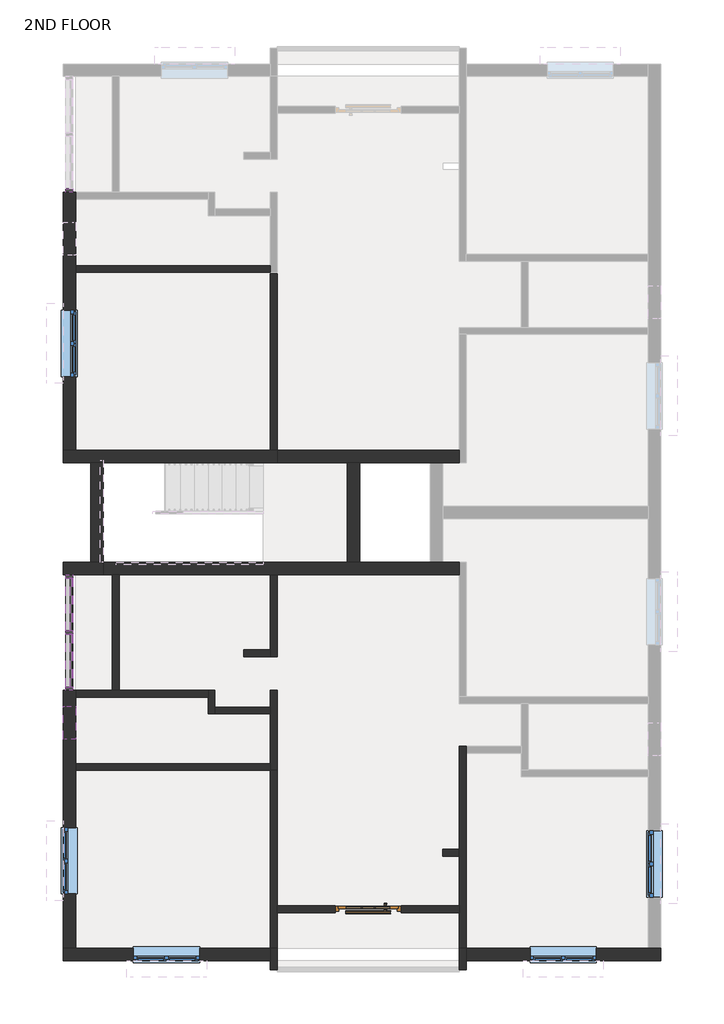
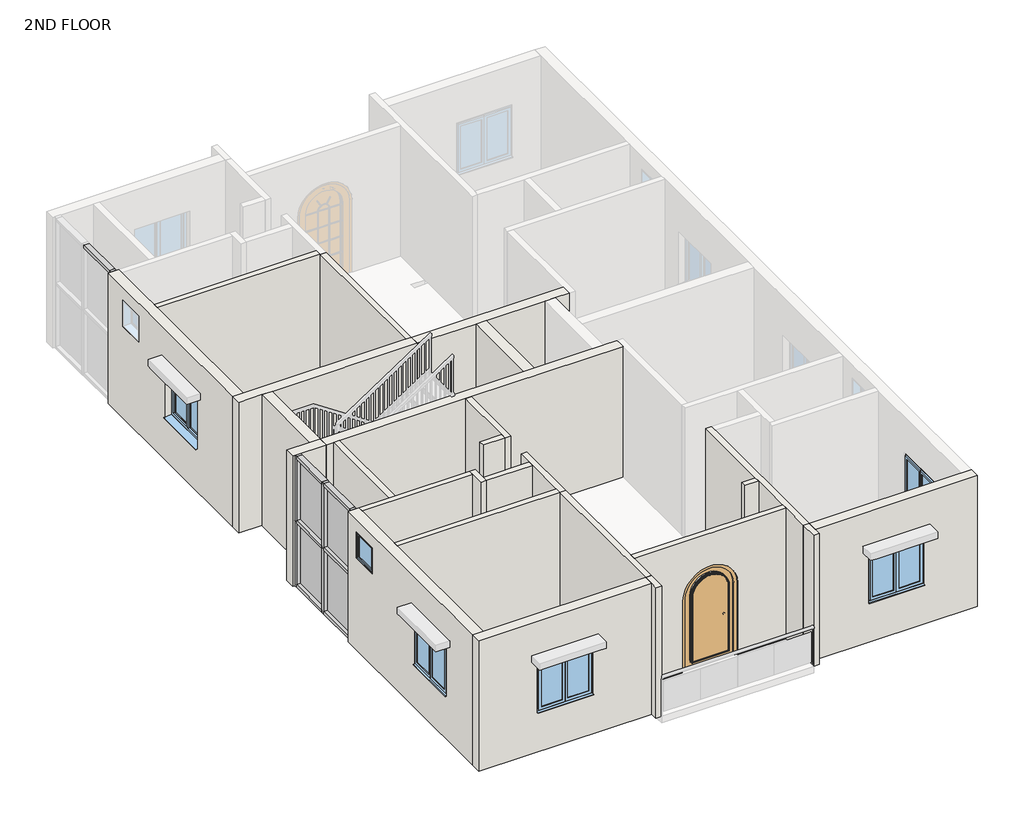
# One storey, part 1 of 4: 26 walls, 15 members, 6 windows, 4 plates, 1 door.
"""IFC4 building model written with IfcOpenShell, lengths in millimetres."""

from ifc_helpers import new_model, si_unit, point, frame, frame_2d, origin, place, context, project, spatial, polyline, circle_curve, trimmed, segment, composite_curve, outline, extrude, faceted_brep, transform, mapped, element, save
from components import door_arched_single_french_glass_wood_exterior_4_x_7_french_5c4dec95, member_801a2072, member_82905deb, member_88aa5c81, member_4491d118, system_panel_glazed_a8655be6, window_80340324, w2_windows_4_x_4_9dec5fc7

model = new_model("IFC4")

# Units and contexts
model_context = context("Model", 3, world=origin())
ifc_project = project(units=[si_unit("LENGTHUNIT", "METRE", prefix="MILLI")], contexts=[model_context])

# Site, building, storey
site = spatial("IfcSite", under=ifc_project)
building = spatial("IfcBuilding", under=site)
storey = spatial("IfcBuildingStorey", under=building, Name="2ND FLOOR", Elevation=9144.0)

# Door
placement = place(None, origin())
door_arched_single_french_glass_wood_exterior_4_x_7_french_shape = door_arched_single_french_glass_wood_exterior_4_x_7_french_5c4dec95(model_context)
element("IfcDoor", 1, ObjectType="Door_Arched_Single_French_Glass_Wood_Exterior : 4' x 7' french door", at=placement, inside=storey, context=model_context, shape_type="MappedRepresentation", body=[
    mapped(door_arched_single_french_glass_wood_exterior_4_x_7_french_shape, transform((-817.6012202, -2286.2690997, 9144.0), x_axis=(-1.0, 0.0, 0.0), y_axis=(0.0, -1.0, 0.0), z_axis=(0.0, 0.0, 1.0))),
])

# Members
member_shape = member_801a2072(model_context)
element("IfcMember", 2, ObjectType="Rectangular Mullion : 2.5\" x 5\" rectangular", at=placement, inside=storey, context=model_context, shape_type="MappedRepresentation", body=[
    mapped(member_shape, transform((-6318.2887202, 10972.5309003, 12192.0), x_axis=(0.0, 0.0, 1.0), y_axis=(-1.0, 0.0, 0.0), z_axis=(0.0, -1.0, 0.0))),
])
element("IfcMember", 3, ObjectType="Rectangular Mullion : 2.5\" x 5\" rectangular", at=placement, inside=storey, context=model_context, shape_type="MappedRepresentation", body=[
    mapped(member_shape, transform((-6318.2887202, 1803.1309003, 12192.0), x_axis=(0.0, 0.0, 1.0), y_axis=(-1.0, 0.0, 0.0), z_axis=(0.0, -1.0, 0.0))),
])
element("IfcMember", 4, ObjectType="Rectangular Mullion : 2.5\" x 5\" rectangular", at=placement, inside=storey, context=model_context, shape_type="MappedRepresentation", body=[
    mapped(member_shape, transform((-6318.2887202, 2838.1809003, 12192.0), x_axis=(0.0, 0.0, 1.0), y_axis=(-1.0, 0.0, 0.0), z_axis=(0.0, -1.0, 0.0))),
])
element("IfcMember", 5, ObjectType="Rectangular Mullion : 2.5\" x 5\" rectangular", at=placement, inside=storey, context=model_context, shape_type="MappedRepresentation", body=[
    mapped(member_shape, transform((-6318.2887202, 3809.7309003, 9144.0), x_axis=(0.0, 0.0, -1.0), y_axis=(-1.0, 0.0, 0.0), z_axis=(0.0, 1.0, 0.0))),
])
element("IfcMember", 6, ObjectType="Rectangular Mullion : 2.5\" x 5\" rectangular", at=placement, inside=storey, context=model_context, shape_type="MappedRepresentation", body=[
    mapped(member_shape, transform((-6318.2887202, 2774.6809003, 9144.0), x_axis=(0.0, 0.0, -1.0), y_axis=(-1.0, 0.0, 0.0), z_axis=(0.0, 1.0, 0.0))),
])
member_2_shape = member_82905deb(model_context)
element("IfcMember", 7, ObjectType="Rectangular Mullion : 2.5\" x 5\" rectangular", at=placement, inside=storey, context=model_context, shape_type="MappedRepresentation", body=[
    mapped(member_2_shape, transform((-6318.2887202, 2806.4309003, 9144.0), x_axis=(0.0, -1.0, 0.0), y_axis=(-1.0, 0.0, 0.0), z_axis=(0.0, 0.0, -1.0))),
])
member_3_shape = member_88aa5c81(model_context)
element("IfcMember", 8, ObjectType="Rectangular Mullion : 2.5\" x 5\" rectangular", at=placement, inside=storey, context=model_context, shape_type="MappedRepresentation", body=[
    mapped(member_3_shape, transform((-6318.2887202, 2838.1809003, 10668.0), x_axis=(0.0, 0.0, 1.0), y_axis=(-1.0, 0.0, 0.0), z_axis=(0.0, -1.0, 0.0))),
])
element("IfcMember", 9, ObjectType="Rectangular Mullion : 2.5\" x 5\" rectangular", at=placement, inside=storey, context=model_context, shape_type="MappedRepresentation", body=[
    mapped(member_3_shape, transform((-6318.2887202, 1803.1309003, 10668.0), x_axis=(0.0, 0.0, 1.0), y_axis=(-1.0, 0.0, 0.0), z_axis=(0.0, -1.0, 0.0))),
])
element("IfcMember", 10, ObjectType="Rectangular Mullion : 2.5\" x 5\" rectangular", at=placement, inside=storey, context=model_context, shape_type="MappedRepresentation", body=[
    mapped(member_2_shape, transform((-6318.2887202, 2806.4309003, 10668.0), x_axis=(0.0, -1.0, 0.0), y_axis=(-1.0, 0.0, 0.0), z_axis=(0.0, 0.0, -1.0))),
])
member_4_shape = member_4491d118(model_context)
element("IfcMember", 11, ObjectType="Rectangular Mullion : 2.5\" x 5\" rectangular", at=placement, inside=storey, context=model_context, shape_type="MappedRepresentation", body=[
    mapped(member_4_shape, transform((-6318.2887202, 10909.0309003, 9144.0), x_axis=(0.0, -1.0, 0.0), y_axis=(-1.0, 0.0, 0.0), z_axis=(0.0, 0.0, -1.0))),
])
element("IfcMember", 12, ObjectType="Rectangular Mullion : 2.5\" x 5\" rectangular", at=placement, inside=storey, context=model_context, shape_type="MappedRepresentation", body=[
    mapped(member_4_shape, transform((-6318.2887202, 1739.6309003, 9144.0), x_axis=(0.0, -1.0, 0.0), y_axis=(-1.0, 0.0, 0.0), z_axis=(0.0, 0.0, -1.0))),
])
element("IfcMember", 13, ObjectType="Rectangular Mullion : 2.5\" x 5\" rectangular", at=placement, inside=storey, context=model_context, shape_type="MappedRepresentation", body=[
    mapped(member_4_shape, transform((-6318.2887202, 3873.2309003, 12192.0), x_axis=(0.0, 1.0, 0.0), y_axis=(-1.0, 0.0, 0.0), z_axis=(0.0, 0.0, 1.0))),
])
element("IfcMember", 14, ObjectType="Rectangular Mullion : 2.5\" x 5\" rectangular", at=placement, inside=storey, context=model_context, shape_type="MappedRepresentation", body=[
    mapped(member_4_shape, transform((-6318.2887202, 10909.0309003, 10668.0), x_axis=(0.0, -1.0, 0.0), y_axis=(-1.0, 0.0, 0.0), z_axis=(0.0, 0.0, -1.0))),
])
element("IfcMember", 15, ObjectType="Rectangular Mullion : 2.5\" x 5\" rectangular", at=placement, inside=storey, context=model_context, shape_type="MappedRepresentation", body=[
    mapped(member_4_shape, transform((-6318.2887202, 1739.6309003, 10668.0), x_axis=(0.0, -1.0, 0.0), y_axis=(-1.0, 0.0, 0.0), z_axis=(0.0, 0.0, -1.0))),
])
element("IfcMember", 16, ObjectType="Rectangular Mullion : 2.5\" x 5\" rectangular", at=placement, inside=storey, context=model_context, shape_type="MappedRepresentation", body=[
    mapped(member_4_shape, transform((-6318.2887202, 3873.2309003, 10668.0), x_axis=(0.0, 1.0, 0.0), y_axis=(-1.0, 0.0, 0.0), z_axis=(0.0, 0.0, 1.0))),
])

# Plates
system_panel_glazed_shape = system_panel_glazed_a8655be6(model_context)
element("IfcPlate", 17, ObjectType="System Panel : Glazed", at=placement, inside=storey, context=model_context, shape_type="MappedRepresentation", body=[
    mapped(system_panel_glazed_shape, transform((-6318.2887202, 3323.9559003, 9207.5), x_axis=(0.0, -1.0, 0.0), y_axis=(1.0, 0.0, 0.0), z_axis=(0.0, 0.0, 1.0))),
])
element("IfcPlate", 18, ObjectType="System Panel : Glazed", at=placement, inside=storey, context=model_context, shape_type="MappedRepresentation", body=[
    mapped(system_panel_glazed_shape, transform((-6318.2887202, 2288.9059003, 9207.5), x_axis=(0.0, -1.0, 0.0), y_axis=(1.0, 0.0, 0.0), z_axis=(0.0, 0.0, 1.0))),
])
element("IfcPlate", 19, ObjectType="System Panel : Glazed", at=placement, inside=storey, context=model_context, shape_type="MappedRepresentation", body=[
    mapped(system_panel_glazed_shape, transform((-6318.2887202, 3323.9559003, 10699.75), x_axis=(0.0, -1.0, 0.0), y_axis=(1.0, 0.0, 0.0), z_axis=(0.0, 0.0, 1.0))),
])
element("IfcPlate", 20, ObjectType="System Panel : Glazed", at=placement, inside=storey, context=model_context, shape_type="MappedRepresentation", body=[
    mapped(system_panel_glazed_shape, transform((-6318.2887202, 2288.9059003, 10699.75), x_axis=(0.0, -1.0, 0.0), y_axis=(1.0, 0.0, 0.0), z_axis=(0.0, 0.0, 1.0))),
])

# Walls
element("IfcWall", 21, ObjectType="OUTER WALL 9\"", at=placement, inside=storey, context=model_context, shape_type="Brep", body=[
    faceted_brep([(-6432.5887202, -3238.7690997, 9144.0), (-2621.0012202, -3238.7690997, 9144.0), (-2621.0012202, -3238.7690997, 12192.0), (-6432.5887202, -3238.7690997, 12192.0), (-5137.1887202, -3238.7690997, 10058.4), (-5137.1887202, -3238.7690997, 11277.6), (-3917.9887202, -3238.7690997, 11277.6), (-3917.9887202, -3238.7690997, 10058.4), (-6432.5887202, -3010.1690997, 9144.0), (-6432.5887202, -3010.1690997, 12192.0), (-6203.9887202, -3010.1690997, 12192.0), (-2621.0012202, -3010.1690997, 12192.0), (-2621.0012202, -3010.1690997, 9144.0), (-6203.9887202, -3010.1690997, 9144.0), (-5137.1887202, -3010.1690997, 10058.4), (-3917.9887202, -3010.1690997, 10058.4), (-3917.9887202, -3010.1690997, 11277.6), (-5137.1887202, -3010.1690997, 11277.6)], [[[0, 1, 2, 3], [4, 5, 6, 7]], [[8, 9, 10, 11, 12, 13], [14, 15, 16, 17]], [[1, 0, 8, 13, 12]], [[3, 2, 11, 10, 9]], [[0, 3, 9, 8]], [[2, 1, 12, 11]], [[5, 4, 14, 17]], [[6, 5, 17, 16]], [[7, 6, 16, 15]], [[4, 7, 15, 14]]]),
])
element("IfcWall", 22, ObjectType="OUTER WALL 9\"", at=placement, inside=storey, context=model_context, shape_type="Brep", body=[
    faceted_brep([(-6203.9887202, -3010.1690997, 12192.0), (-6203.9887202, -3010.1690997, 9144.0), (-6203.9887202, 266.4309003, 9144.0), (-6203.9887202, 393.4309003, 9144.0), (-6203.9887202, 1612.6309003, 9144.0), (-6203.9887202, 1739.6309003, 9144.0), (-6203.9887202, 1739.6309003, 12192.0), (-6203.9887202, 1612.6309003, 12192.0), (-6203.9887202, 393.4309003, 12192.0), (-6203.9887202, 266.4309003, 12192.0), (-6203.9887202, -787.6690997, 11363.2), (-6203.9887202, -787.6690997, 10144.0), (-6203.9887202, -2006.8690997, 10144.0), (-6203.9887202, -2006.8690997, 11363.2), (-6203.9887202, 1447.5309003, 11887.2), (-6203.9887202, 1447.5309003, 11277.6), (-6203.9887202, 837.9309003, 11277.6), (-6203.9887202, 837.9309003, 11887.2), (-6432.5887202, -3010.1690997, 9144.0), (-6432.5887202, -3010.1690997, 12192.0), (-6432.5887202, 1739.6309003, 12192.0), (-6432.5887202, 1739.6309003, 9144.0), (-6432.5887202, -787.6690997, 10144.0), (-6432.5887202, -787.6690997, 11363.2), (-6432.5887202, -2006.8690997, 11363.2), (-6432.5887202, -2006.8690997, 10144.0), (-6432.5887202, 1447.5309003, 11277.6), (-6432.5887202, 1447.5309003, 11887.2), (-6432.5887202, 837.9309003, 11887.2), (-6432.5887202, 837.9309003, 11277.6)], [[[0, 1, 2, 3, 4, 5, 6, 7, 8, 9], [10, 11, 12, 13], [14, 15, 16, 17]], [[18, 19, 20, 21], [22, 23, 24, 25], [26, 27, 28, 29]], [[1, 18, 21, 5, 4, 3, 2]], [[19, 0, 9, 8, 7, 6, 20]], [[1, 0, 19, 18]], [[6, 5, 21, 20]], [[23, 22, 11, 10]], [[24, 23, 10, 13]], [[25, 24, 13, 12]], [[22, 25, 12, 11]], [[15, 14, 27, 26]], [[16, 15, 26, 29]], [[17, 16, 29, 28]], [[14, 17, 28, 27]]]),
])
element("IfcWall", 23, ObjectType="OUTER WALL 9\"", at=placement, inside=storey, context=model_context, shape_type="Brep", body=[
    faceted_brep([(4567.1987798, -3010.1690997, 9144.0), (4338.5987798, -3010.1690997, 9144.0), (985.7987798, -3010.1690997, 9144.0), (985.7987798, -3010.1690997, 12192.0), (4338.5987798, -3010.1690997, 12192.0), (4567.1987798, -3010.1690997, 12192.0), (2166.8987798, -3010.1690997, 10058.4), (3386.0987798, -3010.1690997, 10058.4), (3386.0987798, -3010.1690997, 11277.6), (2166.8987798, -3010.1690997, 11277.6), (4567.1987798, -3238.7690997, 9144.0), (4567.1987798, -3238.7690997, 12192.0), (985.7987798, -3238.7690997, 12192.0), (985.7987798, -3238.7690997, 9144.0), (2166.8987798, -3238.7690997, 10058.4), (2166.8987798, -3238.7690997, 11277.6), (3386.0987798, -3238.7690997, 11277.6), (3386.0987798, -3238.7690997, 10058.4)], [[[0, 1, 2, 3, 4, 5], [6, 7, 8, 9]], [[10, 11, 12, 13], [14, 15, 16, 17]], [[2, 1, 0, 10, 13]], [[5, 4, 3, 12, 11]], [[0, 5, 11, 10]], [[15, 14, 6, 9]], [[16, 15, 9, 8]], [[17, 16, 8, 7]], [[14, 17, 7, 6]], [[3, 2, 13, 12]]]),
])
element("IfcWall", 24, ObjectType="OUTER WALL 9\"", at=placement, inside=storey, context=model_context, shape_type="SweptSolid", body=[
    extrude(outline(polyline([(6159.2309003, 9144.0), (6159.2309003, 12192.0), (10909.0309003, 12192.0), (10909.0309003, 9144.0), (6159.2309003, 9144.0)]), holes=[polyline([(7518.1309003, 11363.2), (7518.1309003, 10144.0), (8737.3309003, 10144.0), (8737.3309003, 11363.2), (7518.1309003, 11363.2)]), polyline([(9753.3309003, 11887.2), (9753.3309003, 11277.6), (10362.9309003, 11277.6), (10362.9309003, 11887.2), (9753.3309003, 11887.2)])]), frame((-6432.5887202, 0.0, 0.0), z_axis=(1.0, 0.0, 0.0), x_axis=(0.0, 1.0, 0.0)), (0.0, 0.0, 1.0), 228.6),
])
element("IfcWall", 25, ObjectType="OUTER WALL 9\"", at=placement, inside=storey, context=model_context, shape_type="Brep", body=[
    faceted_brep([(-6432.5887202, 5930.6309003, 9144.0), (-5923.0012202, 5930.6309003, 9144.0), (-5694.4012202, 5930.6309003, 9144.0), (-2494.0012202, 5930.6309003, 9144.0), (-2494.0012202, 5930.6309003, 12192.0), (-5694.4012202, 5930.6309003, 12192.0), (-5923.0012202, 5930.6309003, 12192.0), (-6432.5887202, 5930.6309003, 12192.0), (-6432.5887202, 6159.2309003, 9144.0), (-6432.5887202, 6159.2309003, 12192.0), (-6203.9887202, 6159.2309003, 12192.0), (-2621.0012202, 6159.2309003, 12192.0), (-2494.0012202, 6159.2309003, 12192.0), (-2494.0012202, 6159.2309003, 9144.0), (-2621.0012202, 6159.2309003, 9144.0), (-6203.9887202, 6159.2309003, 9144.0)], [[[0, 1, 2, 3, 4, 5, 6, 7]], [[8, 9, 10, 11, 12, 13, 14, 15]], [[3, 2, 1, 0, 8, 15, 14, 13]], [[7, 6, 5, 4, 12, 11, 10, 9]], [[0, 7, 9, 8]], [[4, 3, 13, 12]]]),
])
element("IfcWall", 26, ObjectType="OUTER WALL 9\"", at=placement, inside=storey, context=model_context, shape_type="SweptSolid", body=[
    extrude(outline(polyline([(-5923.0012202, 4101.8309003), (-5923.0012202, 5930.6309003), (-5694.4012202, 5930.6309003), (-5694.4012202, 4101.8309003), (-5923.0012202, 4101.8309003)])), frame((0.0, 0.0, 9144.0), z_axis=(0.0, 0.0, 1.0), x_axis=(1.0, 0.0, 0.0)), (0.0, 0.0, 1.0), 3048.0),
])
element("IfcWall", 27, ObjectType="OUTER WALL 9\"", at=placement, inside=storey, context=model_context, shape_type="Brep", body=[
    faceted_brep([(-5694.4012202, 4101.8309003, 9144.0), (-5923.0012202, 4101.8309003, 9144.0), (-6432.5887202, 4101.8309003, 9144.0), (-6432.5887202, 4101.8309003, 12192.0), (-5923.0012202, 4101.8309003, 12192.0), (-5694.4012202, 4101.8309003, 12192.0), (-5694.4012202, 3873.2309003, 9144.0), (-5694.4012202, 3873.2309003, 12192.0), (-6432.5887202, 3873.2309003, 12192.0), (-6432.5887202, 3873.2309003, 9144.0)], [[[0, 1, 2, 3, 4, 5]], [[6, 7, 8, 9]], [[2, 1, 0, 6, 9]], [[5, 4, 3, 8, 7]], [[0, 5, 7, 6]], [[3, 2, 9, 8]]]),
])
element("IfcWall", 28, ObjectType="OUTER WALL 9\"", at=placement, inside=storey, context=model_context, shape_type="Brep", body=[
    faceted_brep([(-5694.4012202, 3873.2309003, 9144.0), (-5529.3012202, 3873.2309003, 9144.0), (-5402.3012202, 3873.2309003, 9144.0), (-2621.0012202, 3873.2309003, 9144.0), (-2494.0012202, 3873.2309003, 9144.0), (858.7987798, 3873.2309003, 9144.0), (858.7987798, 3873.2309003, 12192.0), (-2494.0012202, 3873.2309003, 12192.0), (-2621.0012202, 3873.2309003, 12192.0), (-5402.3012202, 3873.2309003, 12192.0), (-5529.3012202, 3873.2309003, 12192.0), (-5694.4012202, 3873.2309003, 12192.0), (-5694.4012202, 4101.8309003, 9144.0), (-5694.4012202, 4101.8309003, 12192.0), (-1198.6012202, 4101.8309003, 12192.0), (-970.0012202, 4101.8309003, 12192.0), (325.3987798, 4101.8309003, 12192.0), (553.9987798, 4101.8309003, 12192.0), (858.7987798, 4101.8309003, 12192.0), (858.7987798, 4101.8309003, 9144.0), (553.9987798, 4101.8309003, 9144.0), (325.3987798, 4101.8309003, 9144.0), (-970.0012202, 4101.8309003, 9144.0), (-1198.6012202, 4101.8309003, 9144.0)], [[[0, 1, 2, 3, 4, 5, 6, 7, 8, 9, 10, 11]], [[12, 13, 14, 15, 16, 17, 18, 19, 20, 21, 22, 23]], [[5, 4, 3, 2, 1, 0, 12, 23, 22, 21, 20, 19]], [[11, 10, 9, 8, 7, 6, 18, 17, 16, 15, 14, 13]], [[0, 11, 13, 12]], [[6, 5, 19, 18]]]),
])
element("IfcWall", 29, ObjectType="OUTER WALL 9\"", at=placement, inside=storey, context=model_context, shape_type="Brep", body=[
    faceted_brep([(858.7987798, 6159.2309003, 9144.0), (-2494.0012202, 6159.2309003, 9144.0), (-2494.0012202, 6159.2309003, 12192.0), (858.7987798, 6159.2309003, 12192.0), (858.7987798, 5930.6309003, 9144.0), (858.7987798, 5930.6309003, 12192.0), (553.9987798, 5930.6309003, 12192.0), (325.3987798, 5930.6309003, 12192.0), (-970.0012202, 5930.6309003, 12192.0), (-1198.6012202, 5930.6309003, 12192.0), (-2494.0012202, 5930.6309003, 12192.0), (-2494.0012202, 5930.6309003, 9144.0), (-1198.6012202, 5930.6309003, 9144.0), (-970.0012202, 5930.6309003, 9144.0), (325.3987798, 5930.6309003, 9144.0), (553.9987798, 5930.6309003, 9144.0)], [[[0, 1, 2, 3]], [[4, 5, 6, 7, 8, 9, 10, 11, 12, 13, 14, 15]], [[1, 0, 4, 15, 14, 13, 12, 11]], [[3, 2, 10, 9, 8, 7, 6, 5]], [[2, 1, 11, 10]], [[0, 3, 5, 4]]]),
])
element("IfcWall", 30, ObjectType="OUTER WALL 9\"", at=placement, inside=storey, context=model_context, shape_type="SweptSolid", body=[
    extrude(outline(polyline([(-1198.6012202, 4101.8309003), (-1198.6012202, 5930.6309003), (-970.0012202, 5930.6309003), (-970.0012202, 4101.8309003), (-1198.6012202, 4101.8309003)])), frame((0.0, 0.0, 9144.0), z_axis=(0.0, 0.0, 1.0), x_axis=(1.0, 0.0, 0.0)), (0.0, 0.0, 1.0), 3048.0),
])
element("IfcWall", 31, ObjectType="inner wall 5\"", at=placement, inside=storey, context=model_context, shape_type="SweptSolid", body=[
    extrude(outline(polyline([(-6202.4012202, 9562.8309003), (-2621.0012202, 9562.8309003), (-2621.0012202, 9435.8309003), (-6202.4012202, 9435.8309003), (-6202.4012202, 9562.8309003)])), frame((0.0, 0.0, 9144.0), z_axis=(0.0, 0.0, 1.0), x_axis=(1.0, 0.0, 0.0)), (0.0, 0.0, 1.0), 3048.0),
])
element("IfcWall", 32, ObjectType="inner wall 5\"", at=placement, inside=storey, context=model_context, shape_type="SweptSolid", body=[
    extrude(outline(polyline([(-5529.3012202, 1739.6309003), (-5529.3012202, 3873.2309003), (-5402.3012202, 3873.2309003), (-5402.3012202, 1739.6309003), (-5529.3012202, 1739.6309003)])), frame((0.0, 0.0, 9144.0), z_axis=(0.0, 0.0, 1.0), x_axis=(1.0, 0.0, 0.0)), (0.0, 0.0, 1.0), 3048.0),
])
element("IfcWall", 33, ObjectType="inner wall 5\"", at=placement, inside=storey, context=model_context, shape_type="Brep", body=[
    faceted_brep([(-2621.0012202, 3873.2309003, 9144.0), (-2621.0012202, 2488.9309003, 9144.0), (-2621.0012202, 2361.9309003, 9144.0), (-2621.0012202, 2361.9309003, 12192.0), (-2621.0012202, 2488.9309003, 12192.0), (-2621.0012202, 3873.2309003, 12192.0), (-2494.0012202, 3873.2309003, 9144.0), (-2494.0012202, 3873.2309003, 12192.0), (-2494.0012202, 2361.9309003, 12192.0), (-2494.0012202, 2361.9309003, 9144.0)], [[[0, 1, 2, 3, 4, 5]], [[6, 7, 8, 9]], [[2, 1, 0, 6, 9]], [[5, 4, 3, 8, 7]], [[0, 5, 7, 6]], [[3, 2, 9, 8]]]),
])
element("IfcWall", 34, ObjectType="inner wall 5\"", at=placement, inside=storey, context=model_context, shape_type="SweptSolid", body=[
    extrude(outline(polyline([(-3103.6012202, 2488.9309003), (-2621.0012202, 2488.9309003), (-2621.0012202, 2361.9309003), (-3103.6012202, 2361.9309003), (-3103.6012202, 2488.9309003)])), frame((0.0, 0.0, 9144.0), z_axis=(0.0, 0.0, 1.0), x_axis=(1.0, 0.0, 0.0)), (0.0, 0.0, 1.0), 3048.0),
])
element("IfcWall", 35, ObjectType="inner wall 5\"", at=placement, inside=storey, context=model_context, shape_type="Brep", body=[
    faceted_brep([(-6203.9887202, 1612.6309003, 9144.0), (-3764.0012202, 1612.6309003, 9144.0), (-3764.0012202, 1612.6309003, 12192.0), (-6203.9887202, 1612.6309003, 12192.0), (-6203.9887202, 1739.6309003, 9144.0), (-6203.9887202, 1739.6309003, 12192.0), (-5529.3012202, 1739.6309003, 12192.0), (-5402.3012202, 1739.6309003, 12192.0), (-3764.0012202, 1739.6309003, 12192.0), (-3764.0012202, 1739.6309003, 9144.0), (-5402.3012202, 1739.6309003, 9144.0), (-5529.3012202, 1739.6309003, 9144.0)], [[[0, 1, 2, 3]], [[4, 5, 6, 7, 8, 9, 10, 11]], [[1, 0, 4, 11, 10, 9]], [[3, 2, 8, 7, 6, 5]], [[0, 3, 5, 4]], [[2, 1, 9, 8]]]),
])
element("IfcWall", 36, ObjectType="inner wall 5\"", at=placement, inside=storey, context=model_context, shape_type="Brep", body=[
    faceted_brep([(-3764.0012202, 1739.6309003, 9144.0), (-3764.0012202, 1612.6309003, 9144.0), (-3764.0012202, 1307.8309003, 9144.0), (-3764.0012202, 1307.8309003, 12192.0), (-3764.0012202, 1612.6309003, 12192.0), (-3764.0012202, 1739.6309003, 12192.0), (-3637.0012202, 1739.6309003, 9144.0), (-3637.0012202, 1739.6309003, 12192.0), (-3637.0012202, 1434.8309003, 12192.0), (-3637.0012202, 1307.8309003, 12192.0), (-3637.0012202, 1307.8309003, 9144.0), (-3637.0012202, 1434.8309003, 9144.0)], [[[0, 1, 2, 3, 4, 5]], [[6, 7, 8, 9, 10, 11]], [[2, 1, 0, 6, 11, 10]], [[5, 4, 3, 9, 8, 7]], [[0, 5, 7, 6]], [[3, 2, 10, 9]]]),
])
element("IfcWall", 37, ObjectType="inner wall 5\"", at=placement, inside=storey, context=model_context, shape_type="SweptSolid", body=[
    extrude(outline(polyline([(-2621.0012202, 1307.8309003), (-3637.0012202, 1307.8309003), (-3637.0012202, 1434.8309003), (-2621.0012202, 1434.8309003), (-2621.0012202, 1307.8309003)])), frame((0.0, 0.0, 9144.0), z_axis=(0.0, 0.0, 1.0), x_axis=(1.0, 0.0, 0.0)), (0.0, 0.0, 1.0), 3048.0),
])
element("IfcWall", 38, ObjectType="inner wall 5\"", at=placement, inside=storey, context=model_context, shape_type="Brep", body=[
    faceted_brep([(-2621.0012202, 1739.6309003, 9144.0), (-2621.0012202, 1434.8309003, 9144.0), (-2621.0012202, 1307.8309003, 9144.0), (-2621.0012202, 393.4309003, 9144.0), (-2621.0012202, 266.4309003, 9144.0), (-2621.0012202, 266.4309003, 12192.0), (-2621.0012202, 393.4309003, 12192.0), (-2621.0012202, 1307.8309003, 12192.0), (-2621.0012202, 1434.8309003, 12192.0), (-2621.0012202, 1739.6309003, 12192.0), (-2494.0012202, 1739.6309003, 9144.0), (-2494.0012202, 1739.6309003, 12192.0), (-2494.0012202, 266.4309003, 12192.0), (-2494.0012202, 266.4309003, 9144.0)], [[[0, 1, 2, 3, 4, 5, 6, 7, 8, 9]], [[10, 11, 12, 13]], [[4, 3, 2, 1, 0, 10, 13]], [[9, 8, 7, 6, 5, 12, 11]], [[0, 9, 11, 10]], [[5, 4, 13, 12]]]),
])
element("IfcWall", 39, ObjectType="inner wall 5\"", at=placement, inside=storey, context=model_context, shape_type="SweptSolid", body=[
    extrude(outline(polyline([(-6203.9887202, 393.4309003), (-2621.0012202, 393.4309003), (-2621.0012202, 266.4309003), (-6203.9887202, 266.4309003), (-6203.9887202, 393.4309003)])), frame((0.0, 0.0, 9144.0), z_axis=(0.0, 0.0, 1.0), x_axis=(1.0, 0.0, 0.0)), (0.0, 0.0, 1.0), 3048.0),
])
element("IfcWall", 40, ObjectType="inner wall 5\"", at=placement, inside=storey, context=model_context, shape_type="Brep", body=[
    faceted_brep([(-2494.0012202, -3010.1690997, 9144.0), (-2494.0012202, -2349.7690997, 9144.0), (-2494.0012202, -2222.7690997, 9144.0), (-2494.0012202, 266.4309003, 9144.0), (-2494.0012202, 266.4309003, 12192.0), (-2494.0012202, -2222.7690997, 12192.0), (-2494.0012202, -2349.7690997, 12192.0), (-2494.0012202, -3010.1690997, 12192.0), (-2621.0012202, -3010.1690997, 9144.0), (-2621.0012202, -3010.1690997, 12192.0), (-2621.0012202, 266.4309003, 12192.0), (-2621.0012202, 266.4309003, 9144.0)], [[[0, 1, 2, 3, 4, 5, 6, 7]], [[8, 9, 10, 11]], [[3, 2, 1, 0, 8, 11]], [[7, 6, 5, 4, 10, 9]], [[4, 3, 11, 10]], [[0, 7, 9, 8]]]),
])
element("IfcWall", 41, ObjectType="inner wall 5\"", at=placement, inside=storey, context=model_context, shape_type="Brep", body=[
    faceted_brep([(985.7987798, -3010.1690997, 9144.0), (985.7987798, 583.9309003, 9144.0), (985.7987798, 710.9309003, 9144.0), (985.7987798, 710.9309003, 12192.0), (985.7987798, 583.9309003, 12192.0), (985.7987798, -3010.1690997, 12192.0), (858.7987798, -3010.1690997, 9144.0), (858.7987798, -3010.1690997, 12192.0), (858.7987798, -2349.7690997, 12192.0), (858.7987798, -2222.7690997, 12192.0), (858.7987798, -1308.3690997, 12192.0), (858.7987798, -1181.3690997, 12192.0), (858.7987798, 710.9309003, 12192.0), (858.7987798, 710.9309003, 9144.0), (858.7987798, -1181.3690997, 9144.0), (858.7987798, -1308.3690997, 9144.0), (858.7987798, -2222.7690997, 9144.0), (858.7987798, -2349.7690997, 9144.0)], [[[0, 1, 2, 3, 4, 5]], [[6, 7, 8, 9, 10, 11, 12, 13, 14, 15, 16, 17]], [[2, 1, 0, 6, 17, 16, 15, 14, 13]], [[5, 4, 3, 12, 11, 10, 9, 8, 7]], [[3, 2, 13, 12]], [[0, 5, 7, 6]]]),
])
element("IfcWall", 42, ObjectType="inner wall 5\"", at=placement, inside=storey, context=model_context, shape_type="Brep", body=[
    faceted_brep([(-2621.0012202, -3010.1690997, 9144.0), (-2621.0012202, -3238.7690997, 9144.0), (-2621.0012202, -3403.8690997, 9144.0), (-2621.0012202, -3403.8690997, 12192.0), (-2621.0012202, -3238.7690997, 12192.0), (-2621.0012202, -3010.1690997, 12192.0), (-2494.0012202, -3010.1690997, 9144.0), (-2494.0012202, -3010.1690997, 12192.0), (-2494.0012202, -3403.8690997, 12192.0), (-2494.0012202, -3403.8690997, 9144.0)], [[[0, 1, 2, 3, 4, 5]], [[6, 7, 8, 9]], [[2, 1, 0, 6, 9]], [[3, 2, 9, 8]], [[5, 4, 3, 8, 7]], [[0, 5, 7, 6]]]),
])
element("IfcWall", 43, ObjectType="inner wall 5\"", at=placement, inside=storey, context=model_context, shape_type="SweptSolid", body=[
    extrude(outline(composite_curve([segment(polyline([(9144.0, -2494.0012202), (9144.0, -1427.2012202), (10822.6, -1427.2012202)]), True, "CONTINUOUS"), segment(trimmed(circle_curve(frame_2d((10822.6, -817.6012202)), 609.6), [point((10822.6, -1427.2012202))], [point((10822.6, -208.0012202))], True, "CARTESIAN"), True, "CONTINUOUS"), segment(polyline([(10822.6, -208.0012202), (9144.0, -208.0012202), (9144.0, 858.7987798), (12192.0, 858.7987798), (12192.0, -2494.0012202), (9144.0, -2494.0012202)]), True, "CONTINUOUS")], self_intersect=False)), frame((0.0, -2349.7690997, 0.0), z_axis=(0.0, 1.0, 0.0), x_axis=(0.0, 0.0, 1.0)), (0.0, 0.0, 1.0), 127.0),
])
element("IfcWall", 44, ObjectType="inner wall 5\"", at=placement, inside=storey, context=model_context, shape_type="SweptSolid", body=[
    extrude(outline(polyline([(553.9987798, -1181.3690997), (858.7987798, -1181.3690997), (858.7987798, -1308.3690997), (553.9987798, -1308.3690997), (553.9987798, -1181.3690997)])), frame((0.0, 0.0, 9144.0), z_axis=(0.0, 0.0, 1.0), x_axis=(1.0, 0.0, 0.0)), (0.0, 0.0, 1.0), 3048.0),
])
element("IfcWall", 45, ObjectType="inner wall 5\"", at=placement, inside=storey, context=model_context, shape_type="SweptSolid", body=[
    extrude(outline(polyline([(-2621.0012202, 6159.2309003), (-2621.0012202, 9410.4309003), (-2494.0012202, 9410.4309003), (-2494.0012202, 6159.2309003), (-2621.0012202, 6159.2309003)])), frame((0.0, 0.0, 9144.0), z_axis=(0.0, 0.0, 1.0), x_axis=(1.0, 0.0, 0.0)), (0.0, 0.0, 1.0), 3048.0),
])
element("IfcWall", 46, ObjectType="inner wall 5\"", at=placement, inside=storey, context=model_context, shape_type="Brep", body=[
    faceted_brep([(858.7987798, -3010.1690997, 9144.0), (858.7987798, -3403.8690997, 9144.0), (858.7987798, -3403.8690997, 12192.0), (858.7987798, -3010.1690997, 12192.0), (985.7987798, -3010.1690997, 9144.0), (985.7987798, -3010.1690997, 12192.0), (985.7987798, -3238.7690997, 12192.0), (985.7987798, -3403.8690997, 12192.0), (985.7987798, -3403.8690997, 9144.0), (985.7987798, -3238.7690997, 9144.0)], [[[0, 1, 2, 3]], [[4, 5, 6, 7, 8, 9]], [[1, 0, 4, 9, 8]], [[2, 1, 8, 7]], [[3, 2, 7, 6, 5]], [[0, 3, 5, 4]]]),
])

# Windows
window_shape = window_80340324(model_context)
element("IfcWindow", 47, ObjectType="Fixed : 24\" x 24\"", at=placement, inside=storey, context=model_context, shape_type="MappedRepresentation", body=[
    mapped(window_shape, transform((-6318.2887202, 1180.8309003, 10363.2), x_axis=(0.0, 1.0, 0.0), y_axis=(-1.0, 0.0, 0.0), z_axis=(0.0, 0.0, 1.0))),
])
w2_windows_4_x_4_shape = w2_windows_4_x_4_9dec5fc7(model_context)
element("IfcWindow", 48, ObjectType="w2 : windows 4' x 4'", at=placement, inside=storey, context=model_context, shape_type="MappedRepresentation", body=[
    mapped(w2_windows_4_x_4_shape, transform((-4527.5887202, -3124.4690997, 9058.4), x_axis=(1.0, 0.0, 0.0), y_axis=(0.0, 1.0, 0.0), z_axis=(0.0, 0.0, 1.0))),
])
element("IfcWindow", 49, ObjectType="w2 : windows 4' x 4'", at=placement, inside=storey, context=model_context, shape_type="MappedRepresentation", body=[
    mapped(w2_windows_4_x_4_shape, transform((2776.4987798, -3124.4690997, 9058.4), x_axis=(1.0, 0.0, 0.0), y_axis=(0.0, 1.0, 0.0), z_axis=(0.0, 0.0, 1.0))),
])
element("IfcWindow", 50, ObjectType="w2 : windows 4' x 4'", at=placement, inside=storey, context=model_context, shape_type="MappedRepresentation", body=[
    mapped(w2_windows_4_x_4_shape, transform((-6318.2887202, 8127.7309003, 9144.0), x_axis=(0.0, 1.0, 0.0), y_axis=(-1.0, 0.0, 0.0), z_axis=(0.0, 0.0, 1.0))),
])
element("IfcWindow", 51, ObjectType="w2 : windows 4' x 4'", at=placement, inside=storey, context=model_context, shape_type="MappedRepresentation", body=[
    mapped(w2_windows_4_x_4_shape, transform((4452.8987798, -1454.4190997, 9144.0), x_axis=(0.0, -1.0, 0.0), y_axis=(1.0, 0.0, 0.0), z_axis=(0.0, 0.0, 1.0))),
])
element("IfcWindow", 52, ObjectType="w2 : windows 4' x 4'", at=placement, inside=storey, context=model_context, shape_type="MappedRepresentation", body=[
    mapped(w2_windows_4_x_4_shape, transform((-6318.2887202, -1397.2690997, 9144.0), x_axis=(0.0, -1.0, 0.0), y_axis=(1.0, 0.0, 0.0), z_axis=(0.0, 0.0, 1.0))),
])

save(model, "model.ifc")

# Revit data of these elements
# Type "Door_Arched_Single_French_Glass_Wood_Exterior : 4' x 7' french door"
#   Type Mark = "17"
#   Type Comments = "External Single"
#   Operation = "SingleSwingRight"
#   Keynote = "L20"
#   Analytic Construction = "<None>"
#   Wrap Layers (Int) from Ext = 0' - 6.98819"
#   Wrap Layers (Ext) from Ext = 0' - 4.03543"
#   Thickness = 0' - 1.73228"
#   Stile Shutting = 0' - 5.90551"
#   Stile - Top Rail = 0' - 5.90551"
#   Stile - Hanging = 0' - 5.90551"
#   Stile - Bottom Rail = 0' - 6.88976"
#   Rough Width = 4' - 0"
#   Rough Height = 7' - 0"
#   O/A Frame Width = 0' - 2.51969"
#   Handle Z Distance = 3' - 5.33858"
#   Glazing Thickness = 0' - 0.94488"
#   Glazing Bar Thickness = 0' - 0.7874"
#   FrameWidth = 0' - 1.65354"
#   FrameOffset - External = 0' - 0.98425"
#   FrameDepth = 0' - 3.50394"
#   Door Panel Width = 3' - 7.94488"
#   Handle X Distance = 0' - 2.95276"
#   Height = 7' - 0"
#   Structural Tolerance = 0' - 0.25591"
#   Tolerance = 0' - 0.11811"
#   Undercut = 0' - 0.15748"
#   Width = 4' - 0"
#   Door Panel Thickness = 0' - 1.73228"
#   Door Panel Height = 6' - 9.81496"
#   Cavity Closer Width = 0' - 1.9685"
#   Cavity Closer Offset from Ext = 0' - 4.03543"
#   Cavity Closer Depth = 0' - 3.34646"
#   Vis - Ironmongery = yes
#   Vis - Cavity Closers = yes
#   Define Thermal Properties by = 1
#   Material Glass = Door - Glazing
#   Handle Style = element 430241
#   Material Door = Door - Panel
#   Material Frame = BROWN
#   Material Ironmongery = Door - Handle
#   Function = (empty or 0)
#   Wall Closure = (empty or 0)
#   Assembly Code = ""
# Type "Rectangular Mullion : 2.5\" x 5\" rectangular"
#   built-in parameter 1007304 = 0.416667 (stored number, unit not read)
#   built-in parameter 1007301 = 0.104167 (stored number, unit not read)
#   built-in parameter 1007300 = 0.104167 (stored number, unit not read)
# Type "System Panel : Glazed"
#   Construction Type Id = "GSP4R"
#   Analytic Construction = "1/8 in Pilkington single glazing"
#   Visual Light Transmittance = 0.9
#   Solar Heat Gain Coefficient = 0.86
#   Heat Transfer Coefficient (U) = 1.18115 BTU/(h·ft²·°F)
#   Define Thermal Properties by = 1
# Type "OUTER WALL 9\""
#   Assembly Code = "B2010"
#   Layers, outside or top first: 0' - 9" "ROSE COLOUR" (function 1)
# Type "inner wall 5\""
#   Assembly Code = "B2010"
#   Layers, outside or top first: 0' - 5" "ROSE COLOUR" (function 1)
# Type "Fixed : 24\" x 24\""
#   Type Mark = "3"
#   Construction Type Id = "GSP4R"
#   Assembly Code = "B2020100"
#   Analytic Construction = "1/8 in Pilkington single glazing"
#   Visual Light Transmittance = 0.9
#   Solar Heat Gain Coefficient = 0.78
#   Heat Transfer Coefficient (U) = 0.6496 BTU/(h·ft²·°F)
#   Height = 2' - 0"
#   Default Sill Height = 3' - 0"
#   Width = 2' - 0"
#   Window Inset = 0' - 0 3/4"
#   Define Thermal Properties by = 1
#   Define Thermal Properties by = 1
#   Glass Pane Material = Glass
#   Sash Material = Sash
#   Wall Closure = (empty or 0)
# Type "w2 : windows 4' x 4'"
#   Type Mark = "31"
#   Operation = "DoublePanelVertical"
#   Keynote = "16.05.01"
#   Analytic Construction = "<None>"
#   Rough Width = 4' - 0"
#   Rough Height = 4' - 0"
#   Rahmentiefe = 0' - 2.3622"
#   Rahmenhöhe unten = 0' - 3.14961"
#   Rahmehöhe oben = 0' - 3.14961"
#   Rahmenbreite = 0' - 2.3622"
#   Heat Transfer Coefficient (U) = 2.81836 BTU/(h·ft²·°F)
#   Height = 4' - 0"
#   Flügeltiefe = 0' - 2.3622"
#   Flügelbreite = 0' - 2.3622"
#   Einbautiefe (von außen) [instance default] = 0' - 5.51181"
#   Width = 4' - 0"
#   Kippflügel [instance default] = yes
#   Drehflügel im Grundriß darstellen [instance default] = no
#   Drehflügel [instance default] = yes
#   Define Thermal Properties by = 1
#   Rahmen [instance default] = none
#   Glas [instance default] = blue glass
#   Flügel [instance default] = WINDOW COLOUR WHITE
#   Fensterbank aussen [instance default] = WINDOW COLOUR WHITE
#   Fensterbank innen [instance default] = WINDOW COLOUR WHITE
#   Visual Light Transmittance = 0
#   Thermal Resistance (R) = 0
#   Solar Heat Gain Coefficient = 0
#   Wall Closure = (empty or 0)
# Element 1 (IfcDoor, "Door_Arched_Single_French_Glass_Wood_Exterior : 4' x 7' french door")
#   Phase Created = New Construction
#   Materials on its faces: "Door - Panel", "Door - Handle", "BROWN", "Door - Glazing"
# Elements 2, 3, 4, 5, 6, 7, 8, 9, 10, 11, 12, 13, 14, 15, 16 (IfcMember, "Rectangular Mullion : 2.5\" x 5\" rectangular")
#   Phase Created = New Construction
#   Materials on its faces: "Aluminum"
# Elements 17, 18, 19, 20 (IfcPlate, "System Panel : Glazed")
#   Phase Created = New Construction
#   Materials on its faces: "Glass"
# Elements 21, 22, 23, 24, 25, 26, 27, 28, 29, 30 (IfcWall, "OUTER WALL 9\"")
#   Top Offset = 0' - 0"
#   Base Offset = 0' - 0"
#   wall height = 10' - 0"
#   Phase Created = New Construction
#   Base Constraint = 2ND FLOOR
#   Top Constraint = 3RD FLOOR
#   Materials on its faces: "ROSE COLOUR"
# Elements 31, 32, 33, 34, 35, 36, 37, 38, 39, 40, 41, 42, 43, 44, 45, 46 (IfcWall, "inner wall 5\"")
#   Top Offset = 0' - 0"
#   Base Offset = 0' - 0"
#   wall height = 10' - 0"
#   Phase Created = New Construction
#   Base Constraint = 2ND FLOOR
#   Top Constraint = 3RD FLOOR
#   Materials on its faces: "ROSE COLOUR"
# Element 47 (IfcWindow, "Fixed : 24\" x 24\"")
#   Mark = "47"
#   Phase Created = New Construction
#   Materials on its faces: "Sash", "Glass"
# Element 48 (IfcWindow, "w2 : windows 4' x 4'")
#   Mark = "39"
#   Phase Created = New Construction
#   Materials on its faces: "WINDOW COLOUR WHITE", "blue glass"
# Element 49 (IfcWindow, "w2 : windows 4' x 4'")
#   Mark = "40"
#   Phase Created = New Construction
#   Materials on its faces: "WINDOW COLOUR WHITE", "blue glass"
# Element 50 (IfcWindow, "w2 : windows 4' x 4'")
#   Mark = "43"
#   Einbautiefe (von außen) = 0' - 5.51181"
#   Kippflügel = yes
#   Drehflügel im Grundriß darstellen = no
#   Drehflügel = yes
#   Rahmen = none
#   Glas = blue glass
#   Flügel = WINDOW COLOUR WHITE
#   Fensterbank innen = WINDOW COLOUR WHITE
#   Fensterbank aussen = WINDOW COLOUR WHITE
#   Phase Created = New Construction
#   Materials on its faces: "WINDOW COLOUR WHITE", "blue glass"
# Element 51 (IfcWindow, "w2 : windows 4' x 4'")
#   Mark = "44"
#   Einbautiefe (von außen) = 0' - 5.51181"
#   Kippflügel = yes
#   Drehflügel im Grundriß darstellen = no
#   Drehflügel = yes
#   Rahmen = none
#   Glas = blue glass
#   Flügel = WINDOW COLOUR WHITE
#   Fensterbank innen = WINDOW COLOUR WHITE
#   Fensterbank aussen = WINDOW COLOUR WHITE
#   Phase Created = New Construction
#   Materials on its faces: "WINDOW COLOUR WHITE", "blue glass"
# Element 52 (IfcWindow, "w2 : windows 4' x 4'")
#   Mark = "45"
#   Einbautiefe (von außen) = 0' - 5.51181"
#   Kippflügel = yes
#   Drehflügel im Grundriß darstellen = no
#   Drehflügel = yes
#   Rahmen = none
#   Glas = blue glass
#   Flügel = WINDOW COLOUR WHITE
#   Fensterbank innen = WINDOW COLOUR WHITE
#   Fensterbank aussen = WINDOW COLOUR WHITE
#   Phase Created = New Construction
#   Materials on its faces: "WINDOW COLOUR WHITE", "blue glass"
# Materials
#   "Door - Glazing": colour RGB 218 227 224, transparency 0.85
#   "Door - Panel": class "Wood", colour RGB 210 159 95, transparency 0, Cost = 0
#   "BROWN": class "Generic", colour RGB 120 120 120, transparency 0, Cost = 0
#   "Door - Handle": colour RGB 0 0 0, transparency 0, Keynote = "P21"
#   "ROSE COLOUR": class "Generic", colour RGB 120 120 120, transparency 0, Cost = 0
#   "Glass": class "Glass", colour RGB 0 128 192, transparency 0.75, Description = "Soda Lime Glass", Cost = 0
#   "Sash": class "Wood", colour RGB 224 178 126, transparency 0, Cost = 0
#   "blue glass": class "System", colour RGB 0 0 255, transparency 0.75, Cost = 0
#   "WINDOW COLOUR WHITE": class "Generic", colour RGB 120 120 120, transparency 0, Cost = 0
#   "Aluminum": class "Metal", colour RGB 247 247 247, transparency 0, Description = "Aluminum 6061", Cost = 0
